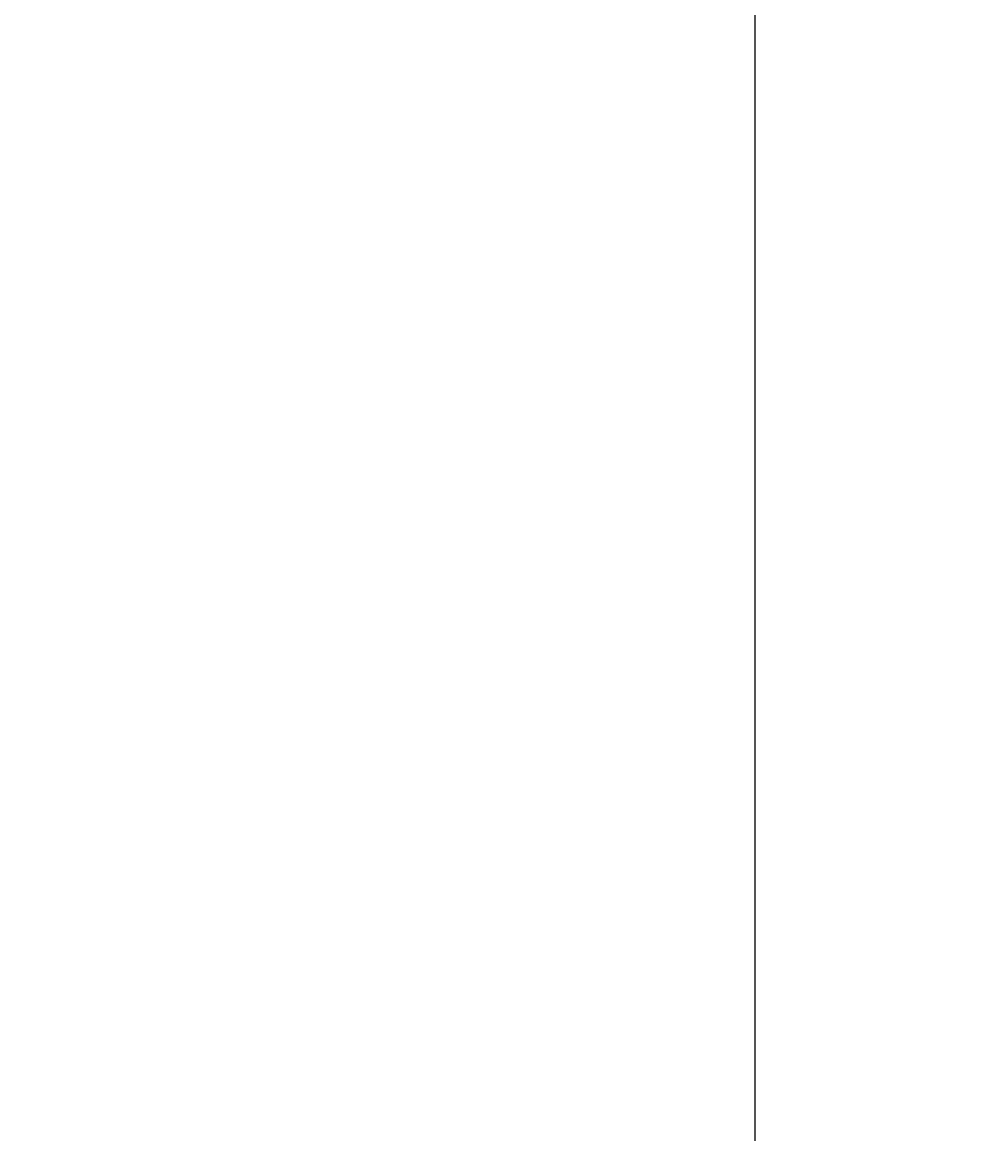
# Model space of a CAD drawing. Units: inches. Extents: x 35362 to 73946, y 43607 to 67532.
# Tile 94 of 134: x 49302 to 50119, y 49735 to 50677. Entities that reach past the tile are written whole.
import ezdxf

# ---------------------------------------------------------------- set-up
doc = ezdxf.new("R2010")
doc.units = ezdxf.units.IN
doc.header["$MEASUREMENT"] = 0
doc.layers.add('A-ANNO-DIMS', color=2, linetype='Continuous', lineweight=18)
doc.styles.get("Standard").update_dxf_attribs({"font": 'arial.ttf'})
doc.dimstyles.get("Standard").update_dxf_attribs({"dimtxt": 0.18, "dimasz": 0.18, "dimexe": 0.18, "dimexo": 0.0625, "dimgap": 0.09, "dimtad": 0, "dimtih": 1, "dimtoh": 1, "dimdec": 4, "dimzin": 0, "dimdsep": 46, "dimtxsty": 'Standard', "dimcen": 0.09, "dimadec": 0, "dimazin": 0, "dimtfac": 1, "dimtdec": 4, "dimtofl": 0, "dimtmove": 0, "dimatfit": 3, "dimfxl": 1, "dimtolj": 1, "dimtzin": 0, "dimarcsym": 0})

# ---------------------------------------------------------------- blocks, each defined once
blk = doc.blocks.new('*D11')
at = {"layer": 'A-ANNO-DIMS', "color": 0, "lineweight": -2, "transparency": 16777216}
for p, q in [((47978.66, 56028.77), (47978.66, 43606.68)), ((53109.76, 56028.77), (53109.76, 43606.68)), ((47978.84, 43606.86), (50543.87, 43606.86)), ((53109.58, 43606.86), (50544.55, 43606.86))]:
    blk.add_line(p, q, dxfattribs=at)
at = {"layer": 'A-ANNO-DIMS', "color": 0, "transparency": 16777216}
for points in [[(47978.84, 43606.89), (47978.84, 43606.83), (47978.66, 43606.86)], [(53109.58, 43606.89), (53109.58, 43606.83), (53109.76, 43606.86)]]:
    blk.add_solid(points, dxfattribs=at)
at = {"layer": 'Defpoints', "color": 0, "transparency": 16777216}
for p in [(47978.66, 56028.84), (53109.76, 56028.84), (53109.76, 43606.86)]:
    blk.add_point(p, dxfattribs=at)
at = {"layer": 'A-ANNO-DIMS', "color": 0, "transparency": 16777216, "insert": (50544.21, 43606.86), "char_height": 0.18, "attachment_point": 5}
blk.add_mtext('\\A1;5131', dxfattribs=at)
blk = doc.blocks.new('*D13')
at = {"layer": 'A-ANNO-DIMS', "color": 0, "lineweight": -2, "transparency": 16777216}
for p, q in [((48373.49, 51694.02), (48373.49, 43606.68)), ((51029.04, 51694.02), (51029.04, 43606.68)), ((48373.67, 43606.86), (49700.8, 43606.86)), ((51028.86, 43606.86), (49701.73, 43606.86))]:
    blk.add_line(p, q, dxfattribs=at)
at = {"layer": 'A-ANNO-DIMS', "color": 0, "transparency": 16777216}
for points in [[(48373.67, 43606.89), (48373.67, 43606.83), (48373.49, 43606.86)], [(51028.86, 43606.89), (51028.86, 43606.83), (51029.04, 43606.86)]]:
    blk.add_solid(points, dxfattribs=at)
at = {"layer": 'Defpoints', "color": 0, "transparency": 16777216}
for p in [(48373.49, 51694.09), (51029.04, 51694.09), (51029.04, 43606.86)]:
    blk.add_point(p, dxfattribs=at)
at = {"layer": 'A-ANNO-DIMS', "color": 0, "transparency": 16777216, "insert": (49701.27, 43606.86), "char_height": 0.18, "attachment_point": 5}
blk.add_mtext('\\A1;2655.6', dxfattribs=at)
blk = doc.blocks.new('*D17')
at = {"layer": 'A-ANNO-DIMS', "color": 0, "lineweight": -2, "transparency": 16777216}
for p, q in [((49923.31, 61293.22), (49923.31, 43606.68)), ((51913.93, 61293.22), (51913.93, 43606.68)), ((49923.49, 43606.86), (50918.16, 43606.86)), ((51913.75, 43606.86), (50919.07, 43606.86))]:
    blk.add_line(p, q, dxfattribs=at)
at = {"layer": 'A-ANNO-DIMS', "color": 0, "transparency": 16777216}
for points in [[(49923.49, 43606.89), (49923.49, 43606.83), (49923.31, 43606.86)], [(51913.75, 43606.89), (51913.75, 43606.83), (51913.93, 43606.86)]]:
    blk.add_solid(points, dxfattribs=at)
at = {"layer": 'Defpoints', "color": 0, "transparency": 16777216}
for p in [(49923.31, 61293.29), (51913.93, 61293.29), (51913.93, 43606.86)]:
    blk.add_point(p, dxfattribs=at)
at = {"layer": 'A-ANNO-DIMS', "color": 0, "transparency": 16777216, "insert": (50918.62, 43606.86), "char_height": 0.18, "attachment_point": 5}
blk.add_mtext('\\A1;1990.6', dxfattribs=at)
blk = doc.blocks.new('*D40')
at = {"layer": 'A-ANNO-DIMS', "color": 0, "lineweight": -2, "transparency": 16777216}
for p, q in [((56873.54, 53351.53), (35361.77, 53351.53)), ((35361.95, 53351.35), (35361.95, 51333.28)), ((35361.95, 49314.85), (35361.95, 51332.92)), ((51806.45, 49314.67), (35361.77, 49314.67))]:
    blk.add_line(p, q, dxfattribs=at)
at = {"layer": 'A-ANNO-DIMS', "color": 0, "transparency": 16777216}
for points in [[(35361.92, 53351.35), (35361.98, 53351.35), (35361.95, 53351.53)], [(35361.92, 49314.85), (35361.98, 49314.85), (35361.95, 49314.67)]]:
    blk.add_solid(points, dxfattribs=at)
at = {"layer": 'Defpoints', "color": 0, "transparency": 16777216}
for p in [(35361.95, 53351.53), (56873.6, 53351.53), (51806.52, 49314.67)]:
    blk.add_point(p, dxfattribs=at)
at = {"layer": 'A-ANNO-DIMS', "color": 0, "transparency": 16777216, "insert": (35361.95, 51333.1), "char_height": 0.18, "attachment_point": 5}
blk.add_mtext('\\A1;4036.9', dxfattribs=at)
blk = doc.blocks.new('*D67')
at = {"layer": 'A-ANNO-DIMS', "color": 0, "lineweight": -2, "transparency": 16777216}
for p, q in [((56873.54, 53351.53), (35361.77, 53351.53)), ((35361.95, 53351.35), (35361.95, 49400.89)), ((35361.95, 45450.07), (35361.95, 49400.53)), ((53793.58, 45449.89), (35361.77, 45449.89))]:
    blk.add_line(p, q, dxfattribs=at)
at = {"layer": 'A-ANNO-DIMS', "color": 0, "transparency": 16777216}
for points in [[(35361.92, 53351.35), (35361.98, 53351.35), (35361.95, 53351.53)], [(35361.92, 45450.07), (35361.98, 45450.07), (35361.95, 45449.89)]]:
    blk.add_solid(points, dxfattribs=at)
at = {"layer": 'Defpoints', "color": 0, "transparency": 16777216}
for p in [(35361.95, 53351.53), (56873.6, 53351.53), (53793.64, 45449.89)]:
    blk.add_point(p, dxfattribs=at)
at = {"layer": 'A-ANNO-DIMS', "color": 0, "transparency": 16777216, "insert": (35361.95, 49400.71), "char_height": 0.18, "attachment_point": 5}
blk.add_mtext('\\A1;7901.6', dxfattribs=at)

msp = doc.modelspace()

# ---------------------------------------------------------------- dimensions: what is measured, and where the dimension line sits
at = {"layer": 'A-ANNO-DIMS'}
for base, p1, p2, override, picture, middle in [((51913.931, 43606.859), (49923.307, 61293.286), (51913.931, 61293.286), {"dimdec": 1, "dimlfac": 1, "dimrnd": 0, "dimzin": 0, "dimdsep": 46, "dimlunit": 2}, '*D17', (50918.619, 43606.859)), ((53109.76, 43606.859), (47978.665, 56028.836), (53109.76, 56028.836), {"dimdec": 0, "dimlfac": 1, "dimrnd": 0, "dimzin": 0, "dimdsep": 46, "dimlunit": 2}, '*D11', (50544.212, 43606.859)), ((51029.043, 43606.859), (48373.492, 51694.087), (51029.043, 51694.087), {"dimdec": 1, "dimlfac": 1, "dimrnd": 0, "dimzin": 0, "dimdsep": 46, "dimlunit": 2}, '*D13', (49701.267, 43606.859))]:
    dim = msp.add_linear_dim(base=base, p1=p1, p2=p2, dimstyle='Standard', override=override, dxfattribs=at)
    dim.commit()
    dim.dimension.update_dxf_attribs({"geometry": picture, "text_midpoint": middle})
for p1, picture, middle in [((51806.517, 49314.669), '*D40', (35361.949, 51333.099)), ((53793.638, 45449.894), '*D67', (35361.949, 49400.712))]:
    dim = msp.add_linear_dim(base=(35361.949, 53351.529), p1=p1, p2=(56873.602, 53351.529), angle=90, dimstyle='Standard', override={"dimdec": 1, "dimlfac": 1, "dimrnd": 0, "dimzin": 0, "dimdsep": 46, "dimlunit": 2}, dxfattribs=at)
    dim.commit()
    dim.dimension.update_dxf_attribs({"geometry": picture, "text_midpoint": middle})

doc.saveas('drawing.dxf')
